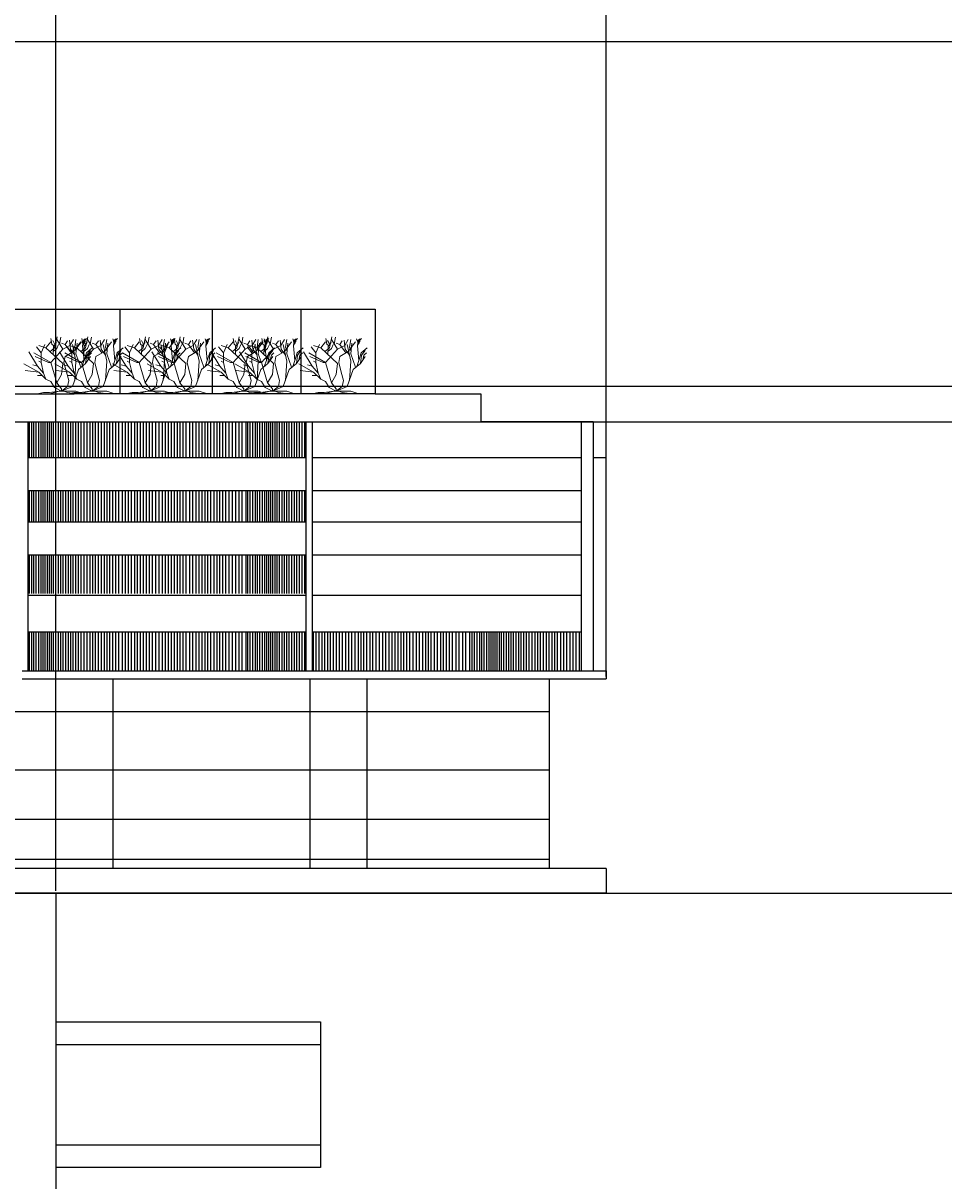
# Model space of a CAD drawing. Units: inches. Extents: x -117 to 121, y -77 to 40.
# Tile 43 of 45: x 72 to 96, y -10 to 21. Entities that reach past the tile are written whole.
import ezdxf

# ---------------------------------------------------------------- set-up
doc = ezdxf.new("R2010")
doc.units = ezdxf.units.IN
doc.header["$MEASUREMENT"] = 0
for name, color, linetype, lineweight in [('A-ANNO-DIMS', 2, 'Continuous', 18), ('A-ELEV', 7, 'Continuous', 25), ('L-PLNT', 3, 'Continuous', 13)]:
    doc.layers.add(name, color=color, linetype=linetype, lineweight=lineweight)
doc.styles.get("Standard").update_dxf_attribs({"font": 'arial.ttf'})
doc.dimstyles.get("Standard").update_dxf_attribs({"dimtxt": 0.18, "dimasz": 0.18, "dimexe": 0.18, "dimexo": 0.0625, "dimgap": 0.09, "dimtad": 0, "dimtih": 1, "dimtoh": 1, "dimdec": 4, "dimzin": 0, "dimdsep": 46, "dimtxsty": 'Standard', "dimcen": 0.09, "dimadec": 0, "dimazin": 0, "dimtfac": 1, "dimtdec": 4, "dimtofl": 0, "dimtmove": 0, "dimatfit": 3, "dimfxl": 1, "dimtolj": 1, "dimtzin": 0, "dimarcsym": 0})

# ---------------------------------------------------------------- blocks, each defined once
blk = doc.blocks.new('*U3')
for p, q in [((-16.8, 16.32), (-18.72, 18.72)), ((-14.88, 18.24), (-17.76, 19.2)), ((-16.8, 16.32), (-15.36, 19.68)), ((-14.88, 18.24), (-12.96, 20.64)), ((-12.471, 19.775), (-12.898, 22.044)), ((-11.677, 19.071), (-12.471, 19.775)), ((-11.28, 19.619), (-12.104, 21.184)), ((-12.043, 15.628), (-11.921, 18.836)), ((-11.921, 18.836), (-10.64, 20.401)), ((-11.433, 18.289), (-10.457, 22.749)), ((-10.579, 18.054), (-9.846, 19.697)), ((-8.16, 17.76), (-10.56, 21.6)), ((-9.48, 19.775), (-8.992, 22.592)), ((-7.2, 19.68), (-8.64, 20.16)), ((-8.16, 17.76), (-5.28, 19.2)), ((-7.2, 19.68), (-6.24, 21.12)), ((-4.8, 16.32), (-7.2, 19.68)), ((-5.086, 17.741), (-5.513, 21.34)), ((-5.28, 19.2), (-3.84, 21.6)), ((-2.88, 12.96), (-4.32, 19.68)), ((-3.84, 16.8), (-0.96, 20.64)), ((-3.377, 18.602), (-2.888, 21.575)), ((-2.766, 16.802), (-3.377, 18.602)), ((-2.88, 15.84), (-2.4, 20.16)), ((-0.508, 21.888), (-0.081, 20.558)), ((-0.203, 19.149), (0.102, 21.34)), ((0.346, 13.203), (-0.203, 19.149)), ((-0.142, 19.384), (0.59, 20.401)), ((-0.02, 20.01), (0.896, 21.105)), ((0.041, 20.714), (1.384, 22.044)), ((0.102, 21.34), (0.835, 21.888)), ((-18.24, 11.04), (-21.755, 16.655)), ((-12.96, 12.48), (-19.68, 16.32)), ((-13.92, 12.48), (-19.2, 14.88)), ((-16.8, 12.48), (-16.8, 16.32)), ((-8.16, 12), (-14.88, 18.24)), ((-13.325, 16.724), (-11.433, 18.289)), ((-12.96, 12.48), (-8.16, 17.76)), ((-11.982, 16.802), (-10.579, 18.054)), ((-7.68, 12.48), (-7.2, 14.88)), ((-7.2, 14.88), (-3.84, 16.8)), ((-3.377, 15.315), (-5.086, 17.819)), ((-0.96, 10.56), (-2.88, 15.84)), ((0.346, 13.203), (1.323, 16.254)), ((0.96, 12), (1.44, 15.36)), ((0.96, 12), (2.88, 14.88)), ((1.323, 16.254), (3.642, 18.289)), ((1.44, 15.36), (2.88, 17.28)), ((1.92, 13.44), (2.4, 15.36)), ((2.4, 15.36), (3.36, 16.32)), ((-17.76, 8.64), (-23.663, 11.961)), ((-18.24, 11.04), (-20.16, 11.52)), ((-15.84, 8.16), (-18.24, 11.04)), ((-16.8, 12.48), (-17.76, 12.96)), ((-15.84, 8.16), (-16.8, 12.48)), ((-12.96, 12.48), (-13.92, 12.48)), ((-10.56, 4.32), (-12.96, 12.48)), ((-8.64, 7.68), (-8.16, 12)), ((-6.72, 8.64), (-7.68, 12.48)), ((-4.32, 2.88), (-1.92, 9.6)), ((-3.36, 5.28), (-2.88, 12.96)), ((-1.92, 9.6), (0.96, 12)), ((-0.48, 10.8), (0.346, 13.203)), ((-17.76, 8.64), (-23.128, 9.222)), ((-16.32, 7.2), (-18.24, 7.2)), ((-14.88, 5.76), (-17.76, 8.64)), ((-14.88, 5.76), (-15.84, 8.16)), ((-12.96, 4.8), (-14.88, 5.76)), ((-11.52, 2.4), (-12.96, 4.8)), ((-10.56, 4.32), (-8.64, 7.68)), ((-5.76, 5.28), (-6.72, 8.64)), ((-6.24, 2.88), (-5.76, 5.28)), ((-15.84, 0.48), (-17.76, 0)), ((-13.44, 0.48), (-15.84, 0.48)), ((-9.6, 0.96), (-13.44, 0.48)), ((-9.6, 0.96), (-12.96, 0)), ((-8.64, 0.96), (-11.52, 2.4)), ((-8.64, 1.92), (-10.56, 4.32)), ((-9.6, 0.96), (-7.68, 0.96)), ((-8.64, 0.96), (-4.32, 2.88)), ((-8.64, 0.96), (-6.24, 2.88)), ((-8.64, 0.96), (-8.64, 1.92)), ((-8.64, 0.96), (-2.88, 0.96)), ((-7.68, 0.96), (-6.24, 0.48)), ((-6.24, 0.48), (-3.36, 0)), ((-2.88, 0.96), (0, 0))]:
    blk.add_line(p, q)
blk = doc.blocks.new('*D12')
at = {"layer": 'A-ANNO-DIMS', "color": 0, "lineweight": -2, "transparency": 16777216}
for p, q in [((72.467, -2.59), (72.467, 38.61)), ((87.242, 3.166), (87.242, 38.61)), ((72.647, 38.43), (79.4, 38.43)), ((87.062, 38.43), (80.309, 38.43))]:
    blk.add_line(p, q, dxfattribs=at)
at = {"layer": 'A-ANNO-DIMS', "color": 0, "transparency": 16777216}
for points in [[(72.647, 38.46), (72.647, 38.4), (72.467, 38.43)], [(87.062, 38.46), (87.062, 38.4), (87.242, 38.43)]]:
    blk.add_solid(points, dxfattribs=at)
at = {"layer": 'Defpoints', "color": 0, "transparency": 16777216}
for p in [(87.242, 38.43), (87.242, 3.104), (72.467, -2.653)]:
    blk.add_point(p, dxfattribs=at)
at = {"layer": 'A-ANNO-DIMS', "color": 0, "transparency": 16777216, "insert": (79.854, 38.43), "char_height": 0.18, "attachment_point": 5}
blk.add_mtext('\\A1;14.774', dxfattribs=at)
blk = doc.blocks.new('*D15')
at = {"layer": 'A-ANNO-DIMS', "color": 0, "lineweight": -2, "transparency": 16777216}
for p, q in [((87.304, -2.653), (120.84, -2.653)), ((120.66, -2.833), (120.66, -20.595)), ((120.66, -38.722), (120.66, -20.959)), ((90.611, -38.902), (120.84, -38.902))]:
    blk.add_line(p, q, dxfattribs=at)
at = {"layer": 'A-ANNO-DIMS', "color": 0, "transparency": 16777216}
for points in [[(120.63, -2.833), (120.69, -2.833), (120.66, -2.653)], [(120.63, -38.722), (120.69, -38.722), (120.66, -38.902)]]:
    blk.add_solid(points, dxfattribs=at)
at = {"layer": 'Defpoints', "color": 0, "transparency": 16777216}
for p in [(87.242, -2.653), (90.549, -38.902), (120.66, -38.902)]:
    blk.add_point(p, dxfattribs=at)
at = {"layer": 'A-ANNO-DIMS', "color": 0, "transparency": 16777216, "insert": (120.66, -20.777), "char_height": 0.18, "attachment_point": 5}
blk.add_mtext('\\A1;36.25', dxfattribs=at)
blk = doc.blocks.new('*D16')
at = {"layer": 'A-ANNO-DIMS', "color": 0, "lineweight": -2, "transparency": 16777216}
for p, q in [((70.862, 21.541), (120.84, 21.541)), ((120.66, 21.361), (120.66, 9.626)), ((120.66, -2.473), (120.66, 9.262)), ((87.304, -2.653), (120.84, -2.653))]:
    blk.add_line(p, q, dxfattribs=at)
at = {"layer": 'A-ANNO-DIMS', "color": 0, "transparency": 16777216}
for points in [[(120.63, 21.361), (120.69, 21.361), (120.66, 21.541)], [(120.63, -2.473), (120.69, -2.473), (120.66, -2.653)]]:
    blk.add_solid(points, dxfattribs=at)
at = {"layer": 'Defpoints', "color": 0, "transparency": 16777216}
for p in [(70.8, 21.541), (87.242, -2.653), (120.66, -2.653)]:
    blk.add_point(p, dxfattribs=at)
at = {"layer": 'A-ANNO-DIMS', "color": 0, "transparency": 16777216, "insert": (120.66, 9.444), "char_height": 0.18, "attachment_point": 5}
blk.add_mtext('\\A1;24.194', dxfattribs=at)
blk = doc.blocks.new('*D24')
at = {"layer": 'A-ANNO-DIMS', "color": 0, "lineweight": -2, "transparency": 16777216}
for p, q in [((87.242, 3.166), (87.242, 38.61)), ((109.85, -61.313), (109.85, 38.61)), ((87.422, 38.43), (98.081, 38.43)), ((109.67, 38.43), (99.011, 38.43))]:
    blk.add_line(p, q, dxfattribs=at)
at = {"layer": 'A-ANNO-DIMS', "color": 0, "transparency": 16777216}
for points in [[(87.422, 38.46), (87.422, 38.4), (87.242, 38.43)], [(109.67, 38.46), (109.67, 38.4), (109.85, 38.43)]]:
    blk.add_solid(points, dxfattribs=at)
at = {"layer": 'Defpoints', "color": 0, "transparency": 16777216}
for p in [(109.85, 38.43), (87.242, 3.104), (109.85, -61.376)]:
    blk.add_point(p, dxfattribs=at)
at = {"layer": 'A-ANNO-DIMS', "color": 0, "transparency": 16777216, "insert": (98.546, 38.43), "char_height": 0.18, "attachment_point": 5}
blk.add_mtext('\\A1;22.609', dxfattribs=at)
blk = doc.blocks.new('*D54')
at = {"layer": 'A-ANNO-DIMS', "color": 0, "lineweight": -2, "transparency": 16777216}
for p, q in [((51.654, 20.218), (120.84, 20.218)), ((120.66, 20.038), (120.66, 15.772)), ((120.66, 11.142), (120.66, 15.408)), ((51.753, 10.962), (120.84, 10.962))]:
    blk.add_line(p, q, dxfattribs=at)
at = {"layer": 'A-ANNO-DIMS', "color": 0, "transparency": 16777216}
for points in [[(120.63, 20.038), (120.69, 20.038), (120.66, 20.218)], [(120.63, 11.142), (120.69, 11.142), (120.66, 10.962)]]:
    blk.add_solid(points, dxfattribs=at)
at = {"layer": 'Defpoints', "color": 0, "transparency": 16777216}
for p in [(51.591, 20.218), (120.66, 20.218), (51.69, 10.962)]:
    blk.add_point(p, dxfattribs=at)
at = {"layer": 'A-ANNO-DIMS', "color": 0, "transparency": 16777216, "insert": (120.66, 15.59), "char_height": 0.18, "attachment_point": 5}
blk.add_mtext('\\A1;9.256', dxfattribs=at)
blk = doc.blocks.new('*D55')
at = {"layer": 'A-ANNO-DIMS', "color": 0, "lineweight": -2, "transparency": 16777216}
for p, q in [((65.473, 10.002), (120.84, 10.002)), ((120.66, 9.822), (120.66, 3.857)), ((120.66, -2.473), (120.66, 3.493)), ((65.624, -2.653), (120.84, -2.653))]:
    blk.add_line(p, q, dxfattribs=at)
at = {"layer": 'A-ANNO-DIMS', "color": 0, "transparency": 16777216}
for points in [[(120.63, 9.822), (120.69, 9.822), (120.66, 10.002)], [(120.63, -2.473), (120.69, -2.473), (120.66, -2.653)]]:
    blk.add_solid(points, dxfattribs=at)
at = {"layer": 'Defpoints', "color": 0, "transparency": 16777216}
for p in [(65.411, 10.002), (120.66, 10.002), (65.562, -2.653)]:
    blk.add_point(p, dxfattribs=at)
at = {"layer": 'A-ANNO-DIMS', "color": 0, "transparency": 16777216, "insert": (120.66, 3.675), "char_height": 0.18, "attachment_point": 5}
blk.add_mtext('\\A1;12.655', dxfattribs=at)

msp = doc.modelspace()

# ---------------------------------------------------------------- linework, layer by layer
at = {"layer": 'A-ELEV'}
for p, q in [((51.6089, 13.0312), (81.0386, 13.0312)), ((74.1866, 13.0312), (74.1866, 10.755)), ((76.6635, 13.0312), (76.6635, 10.755)), ((79.0452, 13.0312), (79.0452, 10.755)), ((81.0386, 13.0312), (81.0386, 10.755)), ((51.6089, 10.755), (72.955, 10.755)), ((81.0386, 10.755), (72.955, 10.755)), ((81.0386, 10.755), (83.882, 10.755)), ((83.882, 10.755), (83.882, 9.9998)), ((65.5651, 9.9998), (83.882, 9.9998)), ((71.7155, 9.9998), (71.7155, 3.3186)), ((71.7569, 9.0454), (71.7569, 9.9998)), ((71.8205, 9.0454), (71.8205, 9.9998)), ((71.878, 9.0454), (71.878, 9.9998)), ((71.9417, 9.0454), (71.9417, 9.9998)), ((72.0113, 9.0454), (72.0113, 9.9998)), ((72.0719, 9.0454), (72.0719, 9.9998)), ((72.1295, 9.0454), (72.1295, 9.9998)), ((72.184, 9.0454), (72.184, 9.9998)), ((72.2385, 9.0454), (72.2385, 9.9998)), ((72.293, 9.0454), (72.293, 9.9998)), ((72.3506, 9.0454), (72.3506, 9.9998)), ((72.4081, 9.0454), (72.4081, 9.9998)), ((72.4691, 9.0454), (72.4691, 9.9998)), ((72.5388, 9.0454), (72.5388, 9.9998)), ((72.6024, 9.0454), (72.6024, 9.9998)), ((72.663, 9.0454), (72.663, 9.9998)), ((72.7326, 9.0454), (72.7326, 9.9998)), ((72.8023, 9.0454), (72.8023, 9.9998)), ((72.8689, 9.0454), (72.8689, 9.9998)), ((72.9325, 9.0454), (72.9325, 9.9998)), ((73.0022, 9.0454), (73.0022, 9.9998)), ((73.0749, 9.0454), (73.0749, 9.9998)), ((73.1476, 9.0454), (73.1476, 9.9998)), ((73.2298, 9.0454), (73.2298, 9.9998)), ((73.3085, 9.0454), (73.3085, 9.9998)), ((73.3842, 9.0454), (73.3842, 9.9998)), ((73.4569, 9.0454), (73.4569, 9.9998)), ((73.5327, 9.0454), (73.5327, 9.9998)), ((73.6118, 9.0454), (73.6118, 9.9998)), ((73.6905, 9.0454), (73.6905, 9.9998)), ((73.7693, 9.0454), (73.7693, 9.9998)), ((73.842, 9.0454), (73.842, 9.9998)), ((73.9147, 9.0454), (73.9147, 9.9998)), ((73.9995, 9.0454), (73.9995, 9.9998)), ((74.0782, 9.0454), (74.0782, 9.9998)), ((74.16, 9.0454), (74.16, 9.9998)), ((74.2544, 9.0454), (74.2544, 9.9998)), ((74.3331, 9.0454), (74.3331, 9.9998)), ((74.4149, 9.0454), (74.4149, 9.9998)), ((74.5027, 9.0454), (74.5027, 9.9998)), ((74.5876, 9.0454), (74.5876, 9.9998)), ((74.6603, 9.0454), (74.6603, 9.9998)), ((74.736, 9.0454), (74.736, 9.9998)), ((74.8178, 9.0454), (74.8178, 9.9998)), ((74.9026, 9.0454), (74.9026, 9.9998)), ((74.9783, 9.0454), (74.9783, 9.9998)), ((75.0665, 9.0454), (75.0665, 9.9998)), ((75.1544, 9.0454), (75.1544, 9.9998)), ((75.2452, 9.0454), (75.2452, 9.9998)), ((75.327, 9.0454), (75.327, 9.9998)), ((75.4149, 9.0454), (75.4149, 9.9998)), ((75.4906, 9.0454), (75.4906, 9.9998)), ((75.5754, 9.0454), (75.5754, 9.9998)), ((75.6572, 9.0454), (75.6572, 9.9998)), ((75.7329, 9.0454), (75.7329, 9.9998)), ((75.8056, 9.0454), (75.8056, 9.9998)), ((75.888, 9.0454), (75.888, 9.9998)), ((75.9698, 9.0454), (75.9698, 9.9998)), ((76.0606, 9.0454), (76.0606, 9.9998)), ((76.1454, 9.0454), (76.1454, 9.9998)), ((76.2303, 9.0454), (76.2303, 9.9998)), ((76.3151, 9.0454), (76.3151, 9.9998)), ((76.3969, 9.0454), (76.3969, 9.9998)), ((76.4726, 9.0454), (76.4726, 9.9998)), ((76.5453, 9.0454), (76.5453, 9.9998)), ((76.6271, 9.0454), (76.6271, 9.9998)), ((76.7149, 9.0454), (76.7149, 9.9998)), ((76.7997, 9.0454), (76.7997, 9.9998)), ((76.8724, 9.0454), (76.8724, 9.9998)), ((76.9512, 9.0454), (76.9512, 9.9998)), ((77.0299, 9.0454), (77.0299, 9.9998)), ((77.1178, 9.0454), (77.1178, 9.9998)), ((77.2087, 9.0454), (77.2087, 9.9998)), ((77.2965, 9.0454), (77.2965, 9.9998)), ((77.3882, 9.0454), (77.3882, 9.9998)), ((77.473, 9.0454), (77.473, 9.9998)), ((77.576, 9.0454), (77.576, 9.9998)), ((77.621, 9.0454), (77.621, 9.9998)), ((77.6863, 9.0454), (77.6863, 9.9998)), ((77.7603, 9.0454), (77.7603, 9.9998)), ((77.8239, 9.0454), (77.8239, 9.9998)), ((77.8815, 9.0454), (77.8815, 9.9998)), ((77.9451, 9.0454), (77.9451, 9.9998)), ((78.0148, 9.0454), (78.0148, 9.9998)), ((78.0753, 9.0454), (78.0753, 9.9998)), ((78.1329, 9.0454), (78.1329, 9.9998)), ((78.1874, 9.0454), (78.1874, 9.9998)), ((78.2419, 9.0454), (78.2419, 9.9998)), ((78.2965, 9.0454), (78.2965, 9.9998)), ((78.354, 9.0454), (78.354, 9.9998)), ((78.4116, 9.0454), (78.4116, 9.9998)), ((78.4725, 9.0454), (78.4725, 9.9998)), ((78.5422, 9.0454), (78.5422, 9.9998)), ((78.6058, 9.0454), (78.6058, 9.9998)), ((78.6664, 9.0454), (78.6664, 9.9998)), ((78.736, 9.0454), (78.736, 9.9998)), ((78.8057, 9.0454), (78.8057, 9.9998)), ((78.8724, 9.0454), (78.8724, 9.9998)), ((78.936, 9.0454), (78.936, 9.9998)), ((79.0056, 9.0454), (79.0056, 9.9998)), ((79.0783, 9.0454), (79.0783, 9.9998)), ((79.151, 9.0454), (79.151, 9.9998)), ((79.177, 9.9998), (79.177, 3.3186)), ((79.3503, 9.9998), (79.3503, 3.3186)), ((86.7485, 9.9998), (83.882, 9.9998)), ((86.5767, 9.9998), (86.5767, 3.3186)), ((86.8978, 9.9998), (86.7485, 9.9998)), ((86.8978, 9.9998), (86.8978, 3.3186)), ((71.7155, 9.0454), (79.177, 9.0454)), ((79.3503, 9.0454), (86.5767, 9.0454)), ((86.8978, 9.0454), (87.2416, 9.0454)), ((87.2416, 3.3186), (87.2416, 9.0454)), ((71.7155, 8.1584), (79.177, 8.1584)), ((71.7569, 7.3208), (71.7569, 8.1584)), ((71.8205, 7.3208), (71.8205, 8.1584)), ((71.878, 7.3208), (71.878, 8.1584)), ((71.9417, 7.3208), (71.9417, 8.1584)), ((72.0113, 7.3208), (72.0113, 8.1584)), ((72.0719, 7.3208), (72.0719, 8.1584)), ((72.1295, 7.3208), (72.1295, 8.1584)), ((72.184, 7.3208), (72.184, 8.1584)), ((72.2385, 7.3208), (72.2385, 8.1584)), ((72.293, 7.3208), (72.293, 8.1584)), ((72.3506, 7.3208), (72.3506, 8.1584)), ((72.4081, 7.3208), (72.4081, 8.1584)), ((72.4691, 7.3208), (72.4691, 8.1584)), ((72.5388, 7.3208), (72.5388, 8.1584)), ((72.6024, 7.3208), (72.6024, 8.1584)), ((72.663, 7.3208), (72.663, 8.1584)), ((72.7326, 7.3208), (72.7326, 8.1584)), ((72.8023, 7.3208), (72.8023, 8.1584)), ((72.8689, 7.3208), (72.8689, 8.1584)), ((72.9325, 7.3208), (72.9325, 8.1584)), ((73.0022, 7.3208), (73.0022, 8.1584)), ((73.0749, 7.3208), (73.0749, 8.1584)), ((73.1476, 7.3208), (73.1476, 8.1584)), ((73.2298, 7.3208), (73.2298, 8.1584)), ((73.3085, 7.3208), (73.3085, 8.1584)), ((73.3842, 7.3208), (73.3842, 8.1584)), ((73.4569, 7.3208), (73.4569, 8.1584)), ((73.5327, 7.3208), (73.5327, 8.1584)), ((73.6118, 7.3208), (73.6118, 8.1584)), ((73.6905, 7.3208), (73.6905, 8.1584)), ((73.7693, 7.3208), (73.7693, 8.1584)), ((73.842, 7.3208), (73.842, 8.1584)), ((73.9147, 7.3208), (73.9147, 8.1584)), ((73.9995, 7.3208), (73.9995, 8.1584)), ((74.0782, 7.3208), (74.0782, 8.1584)), ((74.16, 7.3208), (74.16, 8.1584)), ((74.2544, 7.3208), (74.2544, 8.1584)), ((74.3331, 7.3208), (74.3331, 8.1584)), ((74.4149, 7.3208), (74.4149, 8.1584)), ((74.5027, 7.3208), (74.5027, 8.1584)), ((74.5876, 7.3208), (74.5876, 8.1584)), ((74.6603, 7.3208), (74.6603, 8.1584)), ((74.736, 7.3208), (74.736, 8.1584)), ((74.8178, 7.3208), (74.8178, 8.1584)), ((74.9026, 7.3208), (74.9026, 8.1584)), ((74.9783, 7.3208), (74.9783, 8.1584)), ((75.0665, 7.3208), (75.0665, 8.1584)), ((75.1544, 7.3208), (75.1544, 8.1584)), ((75.2452, 7.3208), (75.2452, 8.1584)), ((75.327, 7.3208), (75.327, 8.1584)), ((75.4149, 7.3208), (75.4149, 8.1584)), ((75.4906, 7.3208), (75.4906, 8.1584)), ((75.5754, 7.3208), (75.5754, 8.1584)), ((75.6572, 7.3208), (75.6572, 8.1584)), ((75.7329, 7.3208), (75.7329, 8.1584)), ((75.8056, 7.3208), (75.8056, 8.1584)), ((75.888, 7.3208), (75.888, 8.1584)), ((75.9698, 7.3208), (75.9698, 8.1584)), ((76.0606, 7.3208), (76.0606, 8.1584)), ((76.1454, 7.3208), (76.1454, 8.1584)), ((76.2303, 7.3208), (76.2303, 8.1584)), ((76.3151, 7.3208), (76.3151, 8.1584)), ((76.3969, 7.3208), (76.3969, 8.1584)), ((76.4726, 7.3208), (76.4726, 8.1584)), ((76.5453, 7.3208), (76.5453, 8.1584)), ((76.6271, 7.3208), (76.6271, 8.1584)), ((76.7149, 7.3208), (76.7149, 8.1584)), ((76.7997, 7.3208), (76.7997, 8.1584)), ((76.8724, 7.3208), (76.8724, 8.1584)), ((76.9512, 7.3208), (76.9512, 8.1584)), ((77.0299, 7.3208), (77.0299, 8.1584)), ((77.1178, 7.3208), (77.1178, 8.1584)), ((77.2087, 7.3208), (77.2087, 8.1584)), ((77.2965, 7.3208), (77.2965, 8.1584)), ((77.3882, 7.3208), (77.3882, 8.1584)), ((77.473, 7.3208), (77.473, 8.1584)), ((77.576, 7.3208), (77.576, 8.1584)), ((77.621, 7.3208), (77.621, 8.1584)), ((77.6863, 7.3208), (77.6863, 8.1584)), ((77.7603, 7.3208), (77.7603, 8.1584)), ((77.8239, 7.3208), (77.8239, 8.1584)), ((77.8815, 7.3208), (77.8815, 8.1584)), ((77.9451, 7.3208), (77.9451, 8.1584)), ((78.0148, 7.3208), (78.0148, 8.1584)), ((78.0753, 7.3208), (78.0753, 8.1584)), ((78.1329, 7.3208), (78.1329, 8.1584)), ((78.1874, 7.3208), (78.1874, 8.1584)), ((78.2419, 7.3208), (78.2419, 8.1584)), ((78.2965, 7.3208), (78.2965, 8.1584)), ((78.354, 7.3208), (78.354, 8.1584)), ((78.4116, 7.3208), (78.4116, 8.1584)), ((78.4725, 7.3208), (78.4725, 8.1584)), ((78.5422, 7.3208), (78.5422, 8.1584)), ((78.6058, 7.3208), (78.6058, 8.1584)), ((78.6664, 7.3208), (78.6664, 8.1584)), ((78.736, 7.3208), (78.736, 8.1584)), ((78.8057, 7.3208), (78.8057, 8.1584)), ((78.8724, 7.3208), (78.8724, 8.1584)), ((78.936, 7.3208), (78.936, 8.1584)), ((79.0056, 7.3208), (79.0056, 8.1584)), ((79.0783, 7.3208), (79.0783, 8.1584)), ((79.151, 7.3208), (79.151, 8.1584)), ((79.3503, 8.1584), (86.5767, 8.1584)), ((71.7155, 7.3208), (79.177, 7.3208)), ((79.3503, 7.3208), (86.5767, 7.3208)), ((71.7155, 6.4338), (79.177, 6.4338)), ((71.7569, 5.3875), (71.7569, 6.4333)), ((71.8205, 5.3875), (71.8205, 6.4333)), ((71.878, 5.3875), (71.878, 6.4333)), ((71.9417, 5.3875), (71.9417, 6.4333)), ((72.0113, 5.3875), (72.0113, 6.4333)), ((72.0719, 5.3875), (72.0719, 6.4333)), ((72.1295, 5.3875), (72.1295, 6.4333)), ((72.184, 5.3875), (72.184, 6.4333)), ((72.2385, 5.3875), (72.2385, 6.4333)), ((72.293, 5.3875), (72.293, 6.4333)), ((72.3506, 5.3875), (72.3506, 6.4333)), ((72.4081, 5.3875), (72.4081, 6.4333)), ((72.4691, 5.3875), (72.4691, 6.4333)), ((72.5388, 5.3875), (72.5388, 6.4333)), ((72.6024, 5.3875), (72.6024, 6.4333)), ((72.663, 5.3875), (72.663, 6.4333)), ((72.7326, 5.3875), (72.7326, 6.4333)), ((72.8023, 5.3875), (72.8023, 6.4333)), ((72.8689, 5.3875), (72.8689, 6.4333)), ((72.9325, 5.3875), (72.9325, 6.4333)), ((73.0022, 5.3875), (73.0022, 6.4333)), ((73.0749, 5.3875), (73.0749, 6.4333)), ((73.1476, 5.3875), (73.1476, 6.4333)), ((73.2298, 5.3875), (73.2298, 6.4333)), ((73.3085, 5.3875), (73.3085, 6.4333)), ((73.3842, 5.3875), (73.3842, 6.4333)), ((73.4569, 5.3875), (73.4569, 6.4333)), ((73.5327, 5.3875), (73.5327, 6.4333)), ((73.6118, 5.3875), (73.6118, 6.4333)), ((73.6905, 5.3875), (73.6905, 6.4333)), ((73.7693, 5.3875), (73.7693, 6.4333)), ((73.842, 5.3875), (73.842, 6.4333)), ((73.9147, 5.3875), (73.9147, 6.4333)), ((73.9995, 5.3875), (73.9995, 6.4333)), ((74.0782, 5.3875), (74.0782, 6.4333)), ((74.16, 5.3875), (74.16, 6.4333)), ((74.2544, 5.3875), (74.2544, 6.4333)), ((74.3331, 5.3875), (74.3331, 6.4333)), ((74.4149, 5.3875), (74.4149, 6.4333)), ((74.5027, 5.3875), (74.5027, 6.4333)), ((74.5876, 5.3875), (74.5876, 6.4333)), ((74.6603, 5.3875), (74.6603, 6.4333)), ((74.736, 5.3875), (74.736, 6.4333)), ((74.8178, 5.3875), (74.8178, 6.4333)), ((74.9026, 5.3875), (74.9026, 6.4333)), ((74.9783, 5.3875), (74.9783, 6.4333)), ((75.0665, 5.3875), (75.0665, 6.4333)), ((75.1544, 5.3875), (75.1544, 6.4333)), ((75.2452, 5.3875), (75.2452, 6.4333)), ((75.327, 5.3875), (75.327, 6.4333)), ((75.4149, 5.3875), (75.4149, 6.4333)), ((75.4906, 5.3875), (75.4906, 6.4333)), ((75.5754, 5.3875), (75.5754, 6.4333)), ((75.6572, 5.3875), (75.6572, 6.4333)), ((75.7329, 5.3875), (75.7329, 6.4333)), ((75.8056, 5.3875), (75.8056, 6.4333)), ((75.888, 5.3875), (75.888, 6.4333)), ((75.9698, 5.3875), (75.9698, 6.4333)), ((76.0606, 5.3875), (76.0606, 6.4333)), ((76.1454, 5.3875), (76.1454, 6.4333)), ((76.2303, 5.3875), (76.2303, 6.4333)), ((76.3151, 5.3875), (76.3151, 6.4333)), ((76.3969, 5.3875), (76.3969, 6.4333)), ((76.4726, 5.3875), (76.4726, 6.4333)), ((76.5453, 5.3875), (76.5453, 6.4333)), ((76.6271, 5.3875), (76.6271, 6.4333)), ((76.7149, 5.3875), (76.7149, 6.4333)), ((76.7997, 5.3875), (76.7997, 6.4333)), ((76.8724, 5.3875), (76.8724, 6.4333)), ((76.9512, 5.3875), (76.9512, 6.4333)), ((77.0299, 5.3875), (77.0299, 6.4333)), ((77.1178, 5.3875), (77.1178, 6.4333)), ((77.2087, 5.3875), (77.2087, 6.4333)), ((77.2965, 5.3875), (77.2965, 6.4333)), ((77.3882, 5.3875), (77.3882, 6.4333)), ((77.473, 5.3875), (77.473, 6.4333)), ((77.576, 5.3875), (77.576, 6.4333)), ((77.621, 5.3875), (77.621, 6.4333)), ((77.6863, 5.3875), (77.6863, 6.4333)), ((77.7603, 5.3875), (77.7603, 6.4333)), ((77.8239, 5.3875), (77.8239, 6.4333)), ((77.8815, 5.3875), (77.8815, 6.4333)), ((77.9451, 5.3875), (77.9451, 6.4333)), ((78.0148, 5.3875), (78.0148, 6.4333)), ((78.0753, 5.3875), (78.0753, 6.4333)), ((78.1329, 5.3875), (78.1329, 6.4333)), ((78.1874, 5.3875), (78.1874, 6.4333)), ((78.2419, 5.3875), (78.2419, 6.4333)), ((78.2965, 5.3875), (78.2965, 6.4333)), ((78.354, 5.3875), (78.354, 6.4333)), ((78.4116, 5.3875), (78.4116, 6.4333)), ((78.4725, 5.3875), (78.4725, 6.4333)), ((78.5422, 5.3875), (78.5422, 6.4333)), ((78.6058, 5.3875), (78.6058, 6.4333)), ((78.6664, 5.3875), (78.6664, 6.4333)), ((78.736, 5.3875), (78.736, 6.4333)), ((78.8057, 5.3875), (78.8057, 6.4333)), ((78.8724, 5.3875), (78.8724, 6.4333)), ((78.936, 5.3875), (78.936, 6.4333)), ((79.0056, 5.3875), (79.0056, 6.4333)), ((79.0783, 5.3875), (79.0783, 6.4333)), ((79.151, 5.3875), (79.151, 6.4333)), ((79.3503, 6.4338), (86.5767, 6.4338)), ((71.7155, 5.3498), (79.177, 5.3498)), ((79.3503, 5.3498), (86.5767, 5.3498)), ((71.7155, 4.3643), (79.177, 4.3643)), ((71.7569, 3.3186), (71.7569, 4.3643)), ((71.8205, 3.3186), (71.8205, 4.3643)), ((71.878, 3.3186), (71.878, 4.3643)), ((71.9417, 3.3186), (71.9417, 4.3643)), ((72.0113, 3.3186), (72.0113, 4.3643)), ((72.0719, 3.3186), (72.0719, 4.3643)), ((72.1295, 3.3186), (72.1295, 4.3643)), ((72.184, 3.3186), (72.184, 4.3643)), ((72.2385, 3.3186), (72.2385, 4.3643)), ((72.293, 3.3186), (72.293, 4.3643)), ((72.3506, 3.3186), (72.3506, 4.3643)), ((72.4081, 3.3186), (72.4081, 4.3643)), ((72.4691, 3.3186), (72.4691, 4.3643)), ((72.5388, 3.3186), (72.5388, 4.3643)), ((72.6024, 3.3186), (72.6024, 4.3643)), ((72.663, 3.3186), (72.663, 4.3643)), ((72.7326, 3.3186), (72.7326, 4.3643)), ((72.8023, 3.3186), (72.8023, 4.3643)), ((72.8689, 3.3186), (72.8689, 4.3643)), ((72.9325, 3.3186), (72.9325, 4.3643)), ((73.0022, 3.3186), (73.0022, 4.3643)), ((73.0749, 3.3186), (73.0749, 4.3643)), ((73.1476, 3.3186), (73.1476, 4.3643)), ((73.2298, 3.3186), (73.2298, 4.3643)), ((73.3085, 3.3186), (73.3085, 4.3643)), ((73.3842, 3.3186), (73.3842, 4.3643)), ((73.4569, 3.3186), (73.4569, 4.3643)), ((73.5327, 3.3186), (73.5327, 4.3643)), ((73.6118, 3.3186), (73.6118, 4.3643)), ((73.6905, 3.3186), (73.6905, 4.3643)), ((73.7693, 3.3186), (73.7693, 4.3643)), ((73.842, 3.3186), (73.842, 4.3643)), ((73.9147, 3.3186), (73.9147, 4.3643)), ((73.9995, 3.3186), (73.9995, 4.3643)), ((74.0782, 3.3186), (74.0782, 4.3643)), ((74.16, 3.3186), (74.16, 4.3643)), ((74.2544, 3.3186), (74.2544, 4.3643)), ((74.3331, 3.3186), (74.3331, 4.3643)), ((74.4149, 3.3186), (74.4149, 4.3643)), ((74.5027, 3.3186), (74.5027, 4.3643)), ((74.5876, 3.3186), (74.5876, 4.3643)), ((74.6603, 3.3186), (74.6603, 4.3643)), ((74.736, 3.3186), (74.736, 4.3643)), ((74.8178, 3.3186), (74.8178, 4.3643)), ((74.9026, 3.3186), (74.9026, 4.3643)), ((74.9783, 3.3186), (74.9783, 4.3643)), ((75.0665, 3.3186), (75.0665, 4.3643)), ((75.1544, 3.3186), (75.1544, 4.3643)), ((75.2452, 3.3186), (75.2452, 4.3643)), ((75.327, 3.3186), (75.327, 4.3643)), ((75.4149, 3.3186), (75.4149, 4.3643)), ((75.4906, 3.3186), (75.4906, 4.3643)), ((75.5754, 3.3186), (75.5754, 4.3643)), ((75.6572, 3.3186), (75.6572, 4.3643)), ((75.7329, 3.3186), (75.7329, 4.3643)), ((75.8056, 3.3186), (75.8056, 4.3643)), ((75.888, 3.3186), (75.888, 4.3643)), ((75.9698, 3.3186), (75.9698, 4.3643)), ((76.0606, 3.3186), (76.0606, 4.3643)), ((76.1454, 3.3186), (76.1454, 4.3643)), ((76.2303, 3.3186), (76.2303, 4.3643)), ((76.3151, 3.3186), (76.3151, 4.3643)), ((76.3969, 3.3186), (76.3969, 4.3643)), ((76.4726, 3.3186), (76.4726, 4.3643)), ((76.5453, 3.3186), (76.5453, 4.3643)), ((76.6271, 3.3186), (76.6271, 4.3643)), ((76.7149, 3.3186), (76.7149, 4.3643)), ((76.7997, 3.3186), (76.7997, 4.3643)), ((76.8724, 3.3186), (76.8724, 4.3643)), ((76.9512, 3.3186), (76.9512, 4.3643)), ((77.0299, 3.3186), (77.0299, 4.3643)), ((77.1178, 3.3186), (77.1178, 4.3643)), ((77.2087, 3.3186), (77.2087, 4.3643)), ((77.2965, 3.3186), (77.2965, 4.3643)), ((77.3882, 3.3186), (77.3882, 4.3643)), ((77.473, 3.3186), (77.473, 4.3643)), ((77.576, 3.3186), (77.576, 4.3643)), ((77.621, 3.3186), (77.621, 4.3643)), ((77.6863, 3.3186), (77.6863, 4.3643)), ((77.7603, 3.3186), (77.7603, 4.3643)), ((77.8239, 3.3186), (77.8239, 4.3643)), ((77.8815, 3.3186), (77.8815, 4.3643)), ((77.9451, 3.3186), (77.9451, 4.3643)), ((78.0148, 3.3186), (78.0148, 4.3643)), ((78.0753, 3.3186), (78.0753, 4.3643)), ((78.1329, 3.3186), (78.1329, 4.3643)), ((78.1874, 3.3186), (78.1874, 4.3643)), ((78.2419, 3.3186), (78.2419, 4.3643)), ((78.2965, 3.3186), (78.2965, 4.3643)), ((78.354, 3.3186), (78.354, 4.3643)), ((78.4116, 3.3186), (78.4116, 4.3643)), ((78.4725, 3.3186), (78.4725, 4.3643)), ((78.5422, 3.3186), (78.5422, 4.3643)), ((78.6058, 3.3186), (78.6058, 4.3643)), ((78.6664, 3.3186), (78.6664, 4.3643)), ((78.736, 3.3186), (78.736, 4.3643)), ((78.8057, 3.3186), (78.8057, 4.3643)), ((78.8724, 3.3186), (78.8724, 4.3643)), ((78.936, 3.3186), (78.936, 4.3643)), ((79.0056, 3.3186), (79.0056, 4.3643)), ((79.0783, 3.3186), (79.0783, 4.3643)), ((79.151, 3.3186), (79.151, 4.3643)), ((79.3503, 4.3643), (86.5767, 4.3643)), ((79.3877, 3.3186), (79.3877, 4.3643)), ((79.4604, 3.3186), (79.4604, 4.3643)), ((79.5361, 3.3186), (79.5361, 4.3643)), ((79.6152, 3.3186), (79.6152, 4.3643)), ((79.6939, 3.3186), (79.6939, 4.3643)), ((79.7727, 3.3186), (79.7727, 4.3643)), ((79.8454, 3.3186), (79.8454, 4.3643)), ((79.9181, 3.3186), (79.9181, 4.3643)), ((80.0029, 3.3186), (80.0029, 4.3643)), ((80.0817, 3.3186), (80.0817, 4.3643)), ((80.1634, 3.3186), (80.1634, 4.3643)), ((80.2578, 3.3186), (80.2578, 4.3643)), ((80.3365, 3.3186), (80.3365, 4.3643)), ((80.4183, 3.3186), (80.4183, 4.3643)), ((80.5062, 3.3186), (80.5062, 4.3643)), ((80.591, 3.3186), (80.591, 4.3643)), ((80.6637, 3.3186), (80.6637, 4.3643)), ((80.7394, 3.3186), (80.7394, 4.3643)), ((80.8212, 3.3186), (80.8212, 4.3643)), ((80.906, 3.3186), (80.906, 4.3643)), ((80.9817, 3.3186), (80.9817, 4.3643)), ((81.07, 3.3186), (81.07, 4.3643)), ((81.1578, 3.3186), (81.1578, 4.3643)), ((81.2487, 3.3186), (81.2487, 4.3643)), ((81.3305, 3.3186), (81.3305, 4.3643)), ((81.4183, 3.3186), (81.4183, 4.3643)), ((81.494, 3.3186), (81.494, 4.3643)), ((81.5788, 3.3186), (81.5788, 4.3643)), ((81.6606, 3.3186), (81.6606, 4.3643)), ((81.7364, 3.3186), (81.7364, 4.3643)), ((81.8091, 3.3186), (81.8091, 4.3643)), ((81.8914, 3.3186), (81.8914, 4.3643)), ((81.9732, 3.3186), (81.9732, 4.3643)), ((82.0641, 3.3186), (82.0641, 4.3643)), ((82.1489, 3.3186), (82.1489, 4.3643)), ((82.2337, 3.3186), (82.2337, 4.3643)), ((82.3185, 3.3186), (82.3185, 4.3643)), ((82.4003, 3.3186), (82.4003, 4.3643)), ((82.476, 3.3186), (82.476, 4.3643)), ((82.5487, 3.3186), (82.5487, 4.3643)), ((82.6305, 3.3186), (82.6305, 4.3643)), ((82.7183, 3.3186), (82.7183, 4.3643)), ((82.8032, 3.3186), (82.8032, 4.3643)), ((82.8759, 3.3186), (82.8759, 4.3643)), ((82.9546, 3.3186), (82.9546, 4.3643)), ((83.0334, 3.3186), (83.0334, 4.3643)), ((83.1212, 3.3186), (83.1212, 4.3643)), ((83.2121, 3.3186), (83.2121, 4.3643)), ((83.2999, 3.3186), (83.2999, 4.3643)), ((83.3916, 3.3186), (83.3916, 4.3643)), ((83.4764, 3.3186), (83.4764, 4.3643)), ((83.5794, 3.3186), (83.5794, 4.3643)), ((83.6449, 3.3186), (83.6449, 4.3643)), ((83.7102, 3.3186), (83.7102, 4.3643)), ((83.7842, 3.3186), (83.7842, 4.3643)), ((83.8478, 3.3186), (83.8478, 4.3643)), ((83.9054, 3.3186), (83.9054, 4.3643)), ((83.969, 3.3186), (83.969, 4.3643)), ((84.0387, 3.3186), (84.0387, 4.3643)), ((84.0993, 3.3186), (84.0993, 4.3643)), ((84.1568, 3.3186), (84.1568, 4.3643)), ((84.2113, 3.3186), (84.2113, 4.3643)), ((84.2659, 3.3186), (84.2659, 4.3643)), ((84.3204, 3.3186), (84.3204, 4.3643)), ((84.3779, 3.3186), (84.3779, 4.3643)), ((84.4355, 3.3186), (84.4355, 4.3643)), ((84.4964, 3.3186), (84.4964, 4.3643)), ((84.5661, 3.3186), (84.5661, 4.3643)), ((84.6297, 3.3186), (84.6297, 4.3643)), ((84.6903, 3.3186), (84.6903, 4.3643)), ((84.76, 3.3186), (84.76, 4.3643)), ((84.8296, 3.3186), (84.8296, 4.3643)), ((84.8963, 3.3186), (84.8963, 4.3643)), ((84.9599, 3.3186), (84.9599, 4.3643)), ((85.0296, 3.3186), (85.0296, 4.3643)), ((85.1023, 3.3186), (85.1023, 4.3643)), ((85.175, 3.3186), (85.175, 4.3643)), ((85.2571, 3.3186), (85.2571, 4.3643)), ((85.3359, 3.3186), (85.3359, 4.3643)), ((85.4116, 3.3186), (85.4116, 4.3643)), ((85.4843, 3.3186), (85.4843, 4.3643)), ((85.56, 3.3186), (85.56, 4.3643)), ((85.6391, 3.3186), (85.6391, 4.3643)), ((85.7179, 3.3186), (85.7179, 4.3643)), ((85.7966, 3.3186), (85.7966, 4.3643)), ((85.8693, 3.3186), (85.8693, 4.3643)), ((85.942, 3.3186), (85.942, 4.3643)), ((86.0268, 3.3186), (86.0268, 4.3643)), ((86.1056, 3.3186), (86.1056, 4.3643)), ((86.1874, 3.3186), (86.1874, 4.3643)), ((86.2817, 3.3186), (86.2817, 4.3643)), ((86.3605, 3.3186), (86.3605, 4.3643)), ((86.4423, 3.3186), (86.4423, 4.3643)), ((86.5301, 3.3186), (86.5301, 4.3643)), ((71.5668, 3.3186), (87.2416, 3.3186)), ((87.2416, 3.3186), (87.2416, 3.1036)), ((71.5668, 3.1036), (87.2416, 3.1036)), ((72.4671, -1.9953), (72.4671, 3.1036)), ((74.0026, -1.9953), (74.0026, 3.1036)), ((79.2917, -1.9953), (79.2917, 3.1036)), ((80.8272, -1.9953), (80.8272, 3.1036)), ((85.7179, 3.1036), (85.7179, -1.9953)), ((65.5651, 2.2251), (85.7179, 2.2251)), ((65.5651, 0.661), (85.7179, 0.661)), ((65.5651, -0.6675), (85.7179, -0.6675)), ((65.5651, -1.7455), (85.7179, -1.7455)), ((87.2416, -1.9953), (65.5651, -1.9953)), ((87.2416, -1.9953), (87.2416, -2.6528)), ((87.2416, -2.6528), (64.6028, -2.6528)), ((72.4671, -2.6528), (72.4671, -41.7053)), ((72.4671, -6.1091), (79.571, -6.1091)), ((79.571, -6.1091), (79.571, -10.0239)), ((72.4671, -6.7165), (79.571, -6.7165)), ((72.4671, -9.4164), (79.571, -9.4164)), ((79.571, -10.0239), (72.4671, -10.0239))]:
    msp.add_line(p, q, dxfattribs=at)

# ---------------------------------------------------------------- block references
at = {"layer": 'L-PLNT', "xscale": 0.0671647796176818, "yscale": 0.0671647796176818, "zscale": 0.0671647796176818}
for p in [(73.2004, 10.7596), (74.0268, 10.7596), (75.5761, 10.7596), (76.5094, 10.7596), (78.0961, 10.7596), (78.8614, 10.7596), (80.5787, 10.7596)]:
    msp.add_blockref('*U3', p, dxfattribs=at)

# ---------------------------------------------------------------- dimensions: what is measured, and where the dimension line sits
at = {"layer": 'A-ANNO-DIMS'}
for base, p1, p2, picture, middle in [((87.241551, 38.429685), (72.467052, -2.65275), (87.241551, 3.103601), '*D12', (79.854301, 38.429685)), ((109.8502, 38.4297), (87.2416, 3.1036), (109.8502, -61.3756), '*D24', (98.5459, 38.4297))]:
    dim = msp.add_linear_dim(base=base, p1=p1, p2=p2, dimstyle='Standard', override={"dimdec": 3, "dimlfac": 1, "dimrnd": 0, "dimzin": 0, "dimdsep": 46, "dimlunit": 2}, dxfattribs=at)
    dim.commit()
    dim.dimension.update_dxf_attribs({"geometry": picture, "text_midpoint": middle})
for base, p1, p2, override, picture, middle in [((120.6602, -2.6528), (70.8, 21.5414), (87.2416, -2.6528), {"dimdec": 3, "dimlfac": 1, "dimrnd": 0, "dimzin": 0, "dimdsep": 46, "dimlunit": 2}, '*D16', (120.6602, 9.4443)), ((120.6602, 20.2181), (51.6901, 10.9623), (51.5915, 20.2181), {"dimdec": 3, "dimlfac": 1, "dimrnd": 0, "dimzin": 0, "dimdsep": 46, "dimlunit": 2}, '*D54', (120.6602, 15.5902)), ((120.6602, 10.0025), (65.562, -2.6528), (65.4109, 10.0025), {"dimdec": 3, "dimlfac": 1, "dimrnd": 0, "dimzin": 0, "dimdsep": 46, "dimlunit": 2}, '*D55', (120.6602, 3.6749)), ((120.6602, -38.9022), (87.2416, -2.6528), (90.5486, -38.9022), {"dimdec": 2, "dimlfac": 1, "dimrnd": 0, "dimzin": 0, "dimdsep": 46, "dimlunit": 2}, '*D15', (120.6602, -20.7775))]:
    dim = msp.add_linear_dim(base=base, p1=p1, p2=p2, angle=90, dimstyle='Standard', override=override, dxfattribs=at)
    dim.commit()
    dim.dimension.update_dxf_attribs({"geometry": picture, "text_midpoint": middle})

doc.saveas('drawing.dxf')
